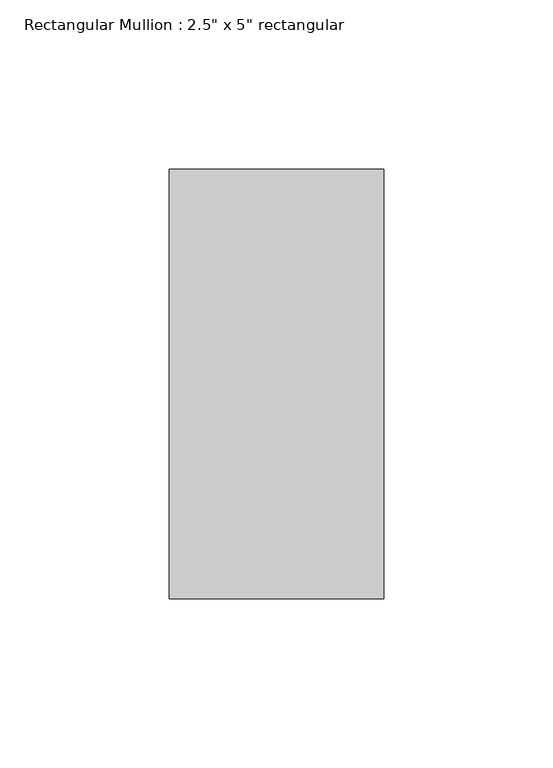
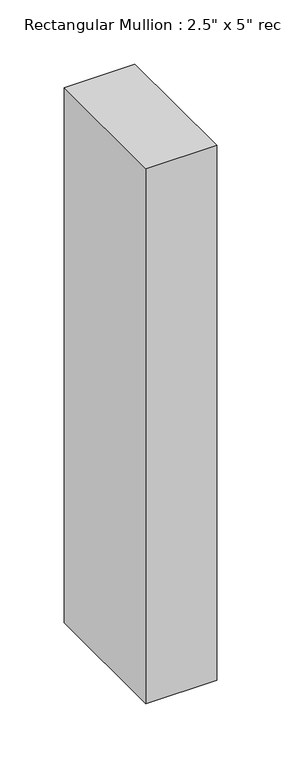
"""IFC4 building model written with IfcOpenShell, lengths in millimetres: member geometry."""

from ifc_helpers import new_model, si_unit, frame, origin, place, context, project, spatial, polyline, outline, extrude, source, transform, mapped, element, save


def member_7fd687a9(model_context):
    return source(origin(), model_context, "Body", "SweptSolid", [
        extrude(outline(polyline([(0.0, 63.5), (0.0, -63.5), (-63.5, -63.5), (-63.5, 63.5), (0.0, 63.5)])), frame((0.0, 0.0, -508.0), z_axis=(0.0, 0.0, 1.0), x_axis=(1.0, 0.0, 0.0)), (0.0, 0.0, 1.0), 508.0),
    ])


if __name__ == "__main__":
    model = new_model("IFC4")
    model_context = context("Model", 3, world=origin())
    ifc_project = project(units=[si_unit("LENGTHUNIT", "METRE", prefix="MILLI")], contexts=[model_context])
    site = spatial("IfcSite", under=ifc_project)
    building = spatial("IfcBuilding", under=site)
    placement = place(None, origin())
    member_shape = member_7fd687a9(model_context)
    element("IfcMember", 1, ObjectType="Rectangular Mullion : 2.5\" x 5\" rectangular", at=placement, inside=building, context=model_context, shape_type="MappedRepresentation", body=[
        mapped(member_shape, transform((0.0, 0.0, 0.0), x_axis=(1.0, 0.0, 0.0), y_axis=(0.0, 1.0, 0.0), z_axis=(0.0, 0.0, 1.0))),
    ])
    save(model, "model.ifc")

# Revit data of these elements
# Type "Rectangular Mullion : 2.5\" x 5\" rectangular"
#   built-in parameter 1007304 = 0.416667 (stored number, unit not read)
#   built-in parameter 1007301 = 0.104167 (stored number, unit not read)
#   built-in parameter 1007300 = 0.104167 (stored number, unit not read)
# Element 1 (IfcMember, "Rectangular Mullion : 2.5\" x 5\" rectangular")
#   Materials on its faces: "Rectangle 1 sq"
# Materials
#   "Rectangle 1 sq": class "Generic", colour RGB 120 120 120, transparency 0, Cost = 0
